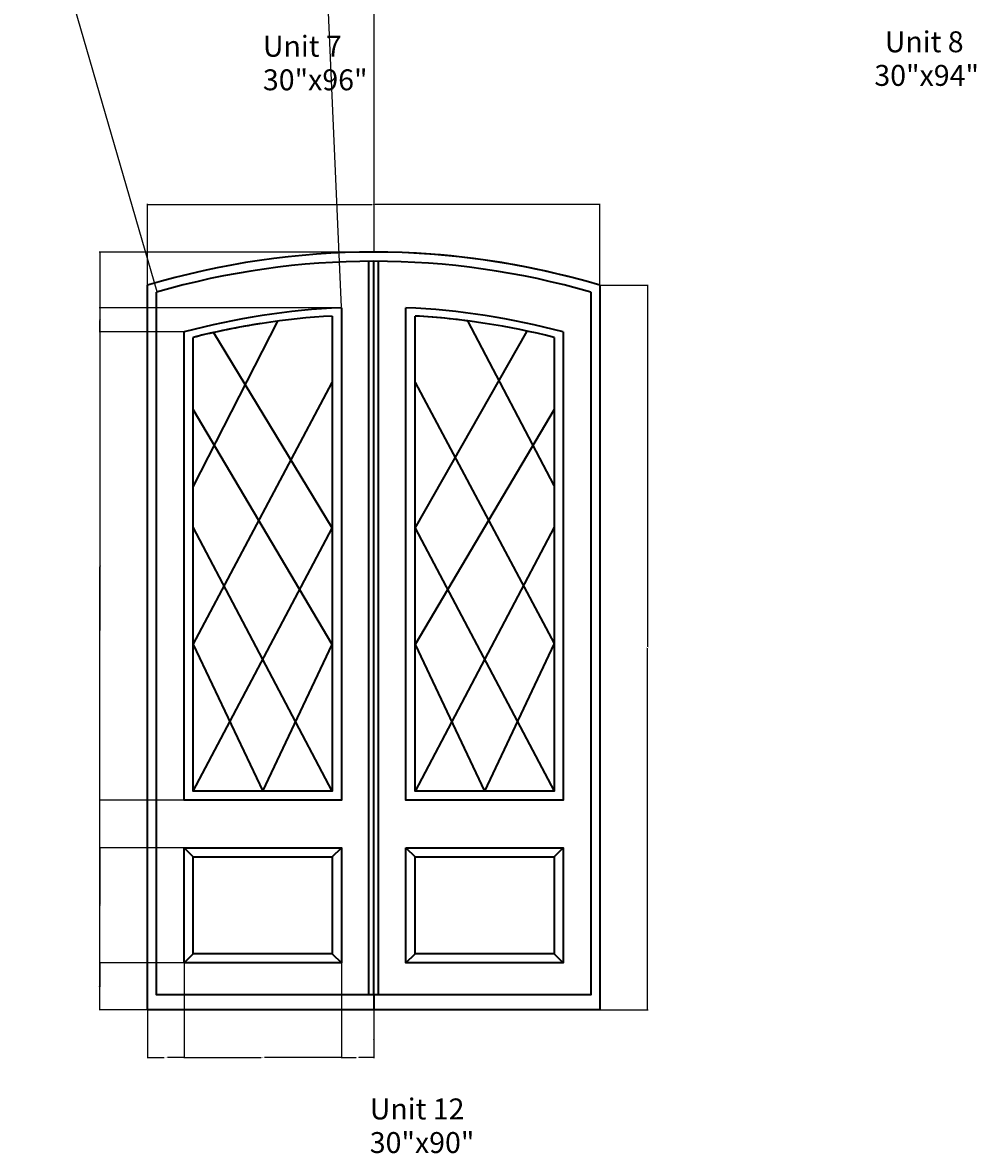
# Model space of a CAD drawing. Units: inches. Extents: x 1318 to 1980, y 617 to 1423.
# Tile 2 of 7: x 1656 to 1930, y 617 to 942. Entities that reach past the tile are written whole.
import ezdxf

# ---------------------------------------------------------------- set-up
doc = ezdxf.new("R2010")
doc.units = ezdxf.units.IN
doc.header["$MEASUREMENT"] = 0
for name, color, linetype, lineweight in [('A-ANNO-DIMS', 2, 'Continuous', 18), ('A-ANNO-TEXT', 7, 'Continuous', 25), ('A-DOOR', 4, 'Continuous', 35)]:
    doc.layers.add(name, color=color, linetype=linetype, lineweight=lineweight)
doc.styles.get("Standard").update_dxf_attribs({"font": 'arial.ttf'})
doc.dimstyles.get("Standard").update_dxf_attribs({"dimtxt": 0.18, "dimasz": 0.18, "dimexe": 0.18, "dimexo": 0.0625, "dimgap": 0.09, "dimtad": 0, "dimtih": 1, "dimtoh": 1, "dimdec": 0, "dimzin": 0, "dimdsep": 46, "dimlunit": 3, "dimtxsty": 'Standard', "dimcen": 0.09, "dimadec": 0, "dimazin": 0, "dimtfac": 1, "dimtdec": 0, "dimtofl": 0, "dimtmove": 0, "dimatfit": 3, "dimfxl": 1, "dimtolj": 1, "dimtzin": 0, "dimarcsym": 0})

# ---------------------------------------------------------------- blocks, each defined once
blk = doc.blocks.new('*D94')
at = {"layer": 'A-ANNO-DIMS', "color": 0, "lineweight": -2, "transparency": 16777216}
for p, q in [((1691.91, 866.32), (1691.91, 889.61)), ((1692.09, 889.43), (1756.33, 889.43)), ((1821.49, 889.43), (1757.24, 889.43)), ((1821.67, 866.32), (1821.67, 889.61))]:
    blk.add_line(p, q, dxfattribs=at)
at = {"layer": 'A-ANNO-DIMS', "color": 0, "transparency": 16777216}
for points in [[(1692.09, 889.46), (1692.09, 889.4), (1691.91, 889.43)], [(1821.49, 889.46), (1821.49, 889.4), (1821.67, 889.43)]]:
    blk.add_solid(points, dxfattribs=at)
at = {"layer": 'Defpoints', "color": 0, "transparency": 16777216}
for p in [(1821.67, 889.43), (1691.91, 866.26), (1821.67, 866.26)]:
    blk.add_point(p, dxfattribs=at)
at = {"layer": 'A-ANNO-DIMS', "color": 0, "transparency": 16777216, "insert": (1756.79, 889.43), "char_height": 0.18, "attachment_point": 5}
blk.add_mtext('\\A1;129.76', dxfattribs=at)
blk = doc.blocks.new('*D95')
at = {"layer": 'A-ANNO-DIMS', "color": 0, "lineweight": -2, "transparency": 16777216}
for p, q in [((1756.72, 875.78), (1678.08, 875.78)), ((1678.26, 875.6), (1678.26, 767.29)), ((1678.26, 658.62), (1678.26, 766.92)), ((1691.85, 658.44), (1678.08, 658.44))]:
    blk.add_line(p, q, dxfattribs=at)
at = {"layer": 'A-ANNO-DIMS', "color": 0, "transparency": 16777216}
for points in [[(1678.23, 875.6), (1678.29, 875.6), (1678.26, 875.78)], [(1678.23, 658.62), (1678.29, 658.62), (1678.26, 658.44)]]:
    blk.add_solid(points, dxfattribs=at)
at = {"layer": 'Defpoints', "color": 0, "transparency": 16777216}
for p in [(1678.26, 875.78), (1756.79, 875.78), (1691.91, 658.44)]:
    blk.add_point(p, dxfattribs=at)
at = {"layer": 'A-ANNO-DIMS', "color": 0, "transparency": 16777216, "insert": (1678.26, 767.11), "char_height": 0.18, "attachment_point": 5}
blk.add_mtext('\\A1;217.34', dxfattribs=at)
blk = doc.blocks.new('*D96')
at = {"layer": 'A-ANNO-DIMS', "color": 0, "lineweight": -2, "transparency": 16777216}
for p, q in [((1747.46, 859.84), (1678.08, 859.84)), ((1678.26, 859.66), (1678.26, 856.54)), ((1678.26, 853.06), (1678.26, 856.18)), ((1702.33, 852.88), (1678.08, 852.88))]:
    blk.add_line(p, q, dxfattribs=at)
at = {"layer": 'A-ANNO-DIMS', "color": 0, "transparency": 16777216}
for points in [[(1678.23, 859.66), (1678.29, 859.66), (1678.26, 859.84)], [(1678.23, 853.06), (1678.29, 853.06), (1678.26, 852.88)]]:
    blk.add_solid(points, dxfattribs=at)
at = {"layer": 'Defpoints', "color": 0, "transparency": 16777216}
for p in [(1678.26, 859.84), (1747.52, 859.84), (1702.4, 852.88)]:
    blk.add_point(p, dxfattribs=at)
at = {"layer": 'A-ANNO-DIMS', "color": 0, "transparency": 16777216, "insert": (1678.26, 856.36), "char_height": 0.18, "attachment_point": 5}
blk.add_mtext('\\A1;6.956', dxfattribs=at)
blk = doc.blocks.new('*D97')
at = {"layer": 'A-ANNO-DIMS', "color": 0, "lineweight": -2, "transparency": 16777216}
for p, q in [((1821.73, 866.26), (1835.5, 866.26)), ((1835.32, 866.08), (1835.32, 762.53)), ((1835.32, 658.62), (1835.32, 762.17)), ((1821.73, 658.44), (1835.5, 658.44))]:
    blk.add_line(p, q, dxfattribs=at)
at = {"layer": 'A-ANNO-DIMS', "color": 0, "transparency": 16777216}
for points in [[(1835.29, 866.08), (1835.35, 866.08), (1835.32, 866.26)], [(1835.29, 658.62), (1835.35, 658.62), (1835.32, 658.44)]]:
    blk.add_solid(points, dxfattribs=at)
at = {"layer": 'Defpoints', "color": 0, "transparency": 16777216}
for p in [(1821.67, 866.26), (1835.32, 866.26), (1821.67, 658.44)]:
    blk.add_point(p, dxfattribs=at)
at = {"layer": 'A-ANNO-DIMS', "color": 0, "transparency": 16777216, "insert": (1835.32, 762.35), "char_height": 0.18, "attachment_point": 5}
blk.add_mtext('\\A1;207.82', dxfattribs=at)
blk = doc.blocks.new('*D98')
at = {"layer": 'A-ANNO-DIMS', "color": 0, "lineweight": -2, "transparency": 16777216}
for p, q in [((1702.4, 671.85), (1702.4, 644.61)), ((1691.91, 658.37), (1691.91, 644.61)), ((1692.09, 644.79), (1696.7, 644.79)), ((1702.22, 644.79), (1697.61, 644.79))]:
    blk.add_line(p, q, dxfattribs=at)
at = {"layer": 'A-ANNO-DIMS', "color": 0, "transparency": 16777216}
for points in [[(1692.09, 644.82), (1692.09, 644.76), (1691.91, 644.79)], [(1702.22, 644.82), (1702.22, 644.76), (1702.4, 644.79)]]:
    blk.add_solid(points, dxfattribs=at)
at = {"layer": 'Defpoints', "color": 0, "transparency": 16777216}
for p in [(1702.4, 671.91), (1691.91, 658.44), (1702.4, 644.79)]:
    blk.add_point(p, dxfattribs=at)
at = {"layer": 'A-ANNO-DIMS', "color": 0, "transparency": 16777216, "insert": (1697.15, 644.79), "char_height": 0.18, "attachment_point": 5}
blk.add_mtext('\\A1;10.488', dxfattribs=at)
blk = doc.blocks.new('*D99')
at = {"layer": 'A-ANNO-DIMS', "color": 0, "lineweight": -2, "transparency": 16777216}
for p, q in [((1702.4, 671.85), (1702.4, 644.61)), ((1747.52, 671.85), (1747.52, 644.61)), ((1702.58, 644.79), (1724.49, 644.79)), ((1747.34, 644.79), (1725.43, 644.79))]:
    blk.add_line(p, q, dxfattribs=at)
at = {"layer": 'A-ANNO-DIMS', "color": 0, "transparency": 16777216}
for points in [[(1702.58, 644.82), (1702.58, 644.76), (1702.4, 644.79)], [(1747.34, 644.82), (1747.34, 644.76), (1747.52, 644.79)]]:
    blk.add_solid(points, dxfattribs=at)
at = {"layer": 'Defpoints', "color": 0, "transparency": 16777216}
for p in [(1702.4, 671.91), (1747.52, 671.91), (1747.52, 644.79)]:
    blk.add_point(p, dxfattribs=at)
at = {"layer": 'A-ANNO-DIMS', "color": 0, "transparency": 16777216, "insert": (1724.96, 644.79), "char_height": 0.18, "attachment_point": 5}
blk.add_mtext('\\A1;45.125', dxfattribs=at)
blk = doc.blocks.new('*D100')
at = {"layer": 'A-ANNO-DIMS', "color": 0, "lineweight": -2, "transparency": 16777216}
for p, q in [((1747.52, 671.85), (1747.52, 644.61)), ((1756.79, 658.37), (1756.79, 644.61)), ((1747.7, 644.79), (1751.76, 644.79)), ((1756.61, 644.79), (1752.55, 644.79))]:
    blk.add_line(p, q, dxfattribs=at)
at = {"layer": 'A-ANNO-DIMS', "color": 0, "transparency": 16777216}
for points in [[(1747.7, 644.82), (1747.7, 644.76), (1747.52, 644.79)], [(1756.61, 644.82), (1756.61, 644.76), (1756.79, 644.79)]]:
    blk.add_solid(points, dxfattribs=at)
at = {"layer": 'Defpoints', "color": 0, "transparency": 16777216}
for p in [(1747.52, 671.91), (1756.79, 658.44), (1756.79, 644.79)]:
    blk.add_point(p, dxfattribs=at)
at = {"layer": 'A-ANNO-DIMS', "color": 0, "transparency": 16777216, "insert": (1752.15, 644.79), "char_height": 0.18, "attachment_point": 5}
blk.add_mtext('\\A1;9.266', dxfattribs=at)
blk = doc.blocks.new('*D101')
at = {"layer": 'A-ANNO-DIMS', "color": 0, "lineweight": -2, "transparency": 16777216}
for p, q in [((1702.33, 671.91), (1678.08, 671.91)), ((1678.26, 671.73), (1678.26, 665.36)), ((1678.26, 658.62), (1678.26, 664.99)), ((1691.85, 658.44), (1678.08, 658.44))]:
    blk.add_line(p, q, dxfattribs=at)
at = {"layer": 'A-ANNO-DIMS', "color": 0, "transparency": 16777216}
for points in [[(1678.23, 671.73), (1678.29, 671.73), (1678.26, 671.91)], [(1678.23, 658.62), (1678.29, 658.62), (1678.26, 658.44)]]:
    blk.add_solid(points, dxfattribs=at)
at = {"layer": 'Defpoints', "color": 0, "transparency": 16777216}
for p in [(1678.26, 671.91), (1702.4, 671.91), (1691.91, 658.44)]:
    blk.add_point(p, dxfattribs=at)
at = {"layer": 'A-ANNO-DIMS', "color": 0, "transparency": 16777216, "insert": (1678.26, 665.17), "char_height": 0.18, "attachment_point": 5}
blk.add_mtext('\\A1;13.477', dxfattribs=at)
blk = doc.blocks.new('*D102')
at = {"layer": 'A-ANNO-DIMS', "color": 0, "lineweight": -2, "transparency": 16777216}
for p, q in [((1702.33, 704.96), (1678.08, 704.96)), ((1678.26, 704.78), (1678.26, 688.62)), ((1678.26, 672.09), (1678.26, 688.25)), ((1702.33, 671.91), (1678.08, 671.91))]:
    blk.add_line(p, q, dxfattribs=at)
at = {"layer": 'A-ANNO-DIMS', "color": 0, "transparency": 16777216}
for points in [[(1678.23, 704.78), (1678.29, 704.78), (1678.26, 704.96)], [(1678.23, 672.09), (1678.29, 672.09), (1678.26, 671.91)]]:
    blk.add_solid(points, dxfattribs=at)
at = {"layer": 'Defpoints', "color": 0, "transparency": 16777216}
for p in [(1678.26, 704.96), (1702.4, 704.96), (1702.4, 671.91)]:
    blk.add_point(p, dxfattribs=at)
at = {"layer": 'A-ANNO-DIMS', "color": 0, "transparency": 16777216, "insert": (1678.26, 688.44), "char_height": 0.18, "attachment_point": 5}
blk.add_mtext('\\A1;33.046', dxfattribs=at)
blk = doc.blocks.new('*D103')
at = {"layer": 'A-ANNO-DIMS', "color": 0, "lineweight": -2, "transparency": 16777216}
for p, q in [((1702.33, 852.88), (1678.08, 852.88)), ((1678.26, 852.7), (1678.26, 785.91)), ((1678.26, 718.75), (1678.26, 785.55)), ((1702.33, 718.57), (1678.08, 718.57))]:
    blk.add_line(p, q, dxfattribs=at)
at = {"layer": 'A-ANNO-DIMS', "color": 0, "transparency": 16777216}
for points in [[(1678.23, 852.7), (1678.29, 852.7), (1678.26, 852.88)], [(1678.23, 718.75), (1678.29, 718.75), (1678.26, 718.57)]]:
    blk.add_solid(points, dxfattribs=at)
at = {"layer": 'Defpoints', "color": 0, "transparency": 16777216}
for p in [(1678.26, 852.88), (1702.4, 852.88), (1702.4, 718.57)]:
    blk.add_point(p, dxfattribs=at)
at = {"layer": 'A-ANNO-DIMS', "color": 0, "transparency": 16777216, "insert": (1678.26, 785.73), "char_height": 0.18, "attachment_point": 5}
blk.add_mtext('\\A1;134.3', dxfattribs=at)
blk = doc.blocks.new('*D118')
at = {"layer": 'A-ANNO-DIMS', "color": 0, "lineweight": -2, "transparency": 16777216}
for p, q in [((1756.97, 1011.3), (1756.79, 1011.3)), ((1756.79, 1011.3), (1756.79, 875.96)), ((1756.7, 649.9), (1756.88, 649.9)), ((1756.79, 649.81), (1756.79, 649.99))]:
    blk.add_line(p, q, dxfattribs=at)
at = {"layer": 'A-ANNO-DIMS', "color": 0, "transparency": 16777216}
blk.add_solid([(1756.76, 875.96), (1756.82, 875.96), (1756.79, 875.78)], dxfattribs=at)
at = {"layer": 'Defpoints', "color": 0, "transparency": 16777216}
for p in [(1756.79, 875.78), (1756.79, 649.9)]:
    blk.add_point(p, dxfattribs=at)
at = {"layer": 'A-ANNO-DIMS', "color": 0, "transparency": 16777216, "insert": (1757.45, 1011.3), "char_height": 0.18, "attachment_point": 5}
blk.add_mtext('\\A1;R225.9', dxfattribs=at)
blk = doc.blocks.new('*D119')
at = {"layer": 'A-ANNO-DIMS', "color": 0, "lineweight": -2, "transparency": 16777216}
for p, q in [((1657.1, 992.97), (1657.28, 992.97)), ((1657.28, 992.97), (1694.55, 864.49)), ((1756.7, 649.9), (1756.88, 649.9)), ((1756.79, 649.81), (1756.79, 649.99))]:
    blk.add_line(p, q, dxfattribs=at)
at = {"layer": 'A-ANNO-DIMS', "color": 0, "transparency": 16777216}
blk.add_solid([(1694.57, 864.5), (1694.52, 864.48), (1694.6, 864.32)], dxfattribs=at)
at = {"layer": 'Defpoints', "color": 0, "transparency": 16777216}
for p in [(1694.6, 864.32), (1756.79, 649.9)]:
    blk.add_point(p, dxfattribs=at)
at = {"layer": 'A-ANNO-DIMS', "color": 0, "transparency": 16777216, "insert": (1656.55, 992.97), "char_height": 0.18, "attachment_point": 5}
blk.add_mtext('\\A1;R223.26', dxfattribs=at)
blk = doc.blocks.new('*D120')
at = {"layer": 'A-ANNO-DIMS', "color": 0, "lineweight": -2, "transparency": 16777216}
for p, q in [((1741.75, 985.8), (1741.93, 985.8)), ((1741.93, 985.8), (1747.49, 860.02)), ((1756.7, 649.9), (1756.88, 649.9)), ((1756.79, 649.81), (1756.79, 649.99))]:
    blk.add_line(p, q, dxfattribs=at)
at = {"layer": 'A-ANNO-DIMS', "color": 0, "transparency": 16777216}
blk.add_solid([(1747.52, 860.02), (1747.46, 860.02), (1747.5, 859.84)], dxfattribs=at)
at = {"layer": 'Defpoints', "color": 0, "transparency": 16777216}
for p in [(1747.5, 859.84), (1756.79, 649.9)]:
    blk.add_point(p, dxfattribs=at)
at = {"layer": 'A-ANNO-DIMS', "color": 0, "transparency": 16777216, "insert": (1741, 985.8), "char_height": 0.18, "attachment_point": 5}
blk.add_mtext('\\A1;4X R210.15', dxfattribs=at)

msp = doc.modelspace()

# ---------------------------------------------------------------- linework, layer by layer
at = {"layer": 'A-DOOR'}
for p, q in [((1755.3874, 662.7536), (1755.3874, 873.1492)), ((1756.7874, 662.7536), (1756.7874, 873.1536)), ((1758.1875, 662.7536), (1758.1875, 873.1492)), ((1705.0189, 808.4828), (1729.2992, 855.9901)), ((1768.6751, 796.5833), (1800.8603, 853.1222)), ((1808.5559, 808.8309), (1783.7627, 856.0572)), ((1710.8281, 852.7085), (1744.8997, 796.5833)), ((1705.0189, 763.193), (1744.8997, 838.3489)), ((1768.6751, 838.3489), (1808.5559, 763.5027)), ((1744.8997, 763.193), (1705.0189, 830.6119)), ((1808.5559, 830.6119), (1768.6751, 763.193)), ((1744.8997, 721.1955), (1705.0189, 796.9217)), ((1705.0189, 721.1955), (1744.8997, 796.5833)), ((1808.5559, 796.9217), (1768.6751, 721.1955)), ((1768.6751, 796.5833), (1808.5559, 721.1955)), ((1705.0189, 763.193), (1724.9593, 721.1955)), ((1724.9593, 721.1955), (1744.8997, 763.193)), ((1768.6751, 763.193), (1788.6155, 721.1955)), ((1808.5559, 763.5027), (1788.6155, 721.1955)), ((1702.397, 704.9593), (1705.0189, 702.3374)), ((1744.8997, 702.3374), (1747.5217, 704.9593)), ((1766.0532, 704.9593), (1768.6751, 702.3374)), ((1808.5559, 702.3374), (1811.1778, 704.9593)), ((1702.397, 671.9133), (1705.0189, 674.5352)), ((1744.8997, 674.5352), (1747.5217, 671.9133)), ((1766.0532, 671.9133), (1768.6751, 674.5352)), ((1808.5559, 674.5352), (1811.1778, 671.9133)), ((1756.7874, 662.7536), (1756.7874, 658.4362))]:
    msp.add_line(p, q, dxfattribs=at)
for points in [[(1821.6654, 866.2577), (1821.6654, 658.4362), (1691.9094, 658.4362), (1691.9094, 866.2577)], [(1819.0435, 864.2978), (1819.0435, 662.7536), (1694.5313, 662.7536), (1694.5313, 864.2978)], [(1747.5217, 859.8397), (1747.5217, 718.5736), (1702.397, 718.5736), (1702.397, 852.8834)], [(1811.1778, 852.8834), (1811.1778, 718.5736), (1766.0532, 718.5736), (1766.0532, 859.8397)], [(1744.8997, 857.4592), (1744.8997, 721.1955), (1705.0189, 721.1955), (1705.0189, 851.3195)], [(1808.5559, 851.3195), (1808.5559, 721.1955), (1768.6751, 721.1955), (1768.6751, 857.4592)]]:
    msp.add_lwpolyline(points, dxfattribs=at)
for points in [[(1702.397, 704.9593), (1747.5217, 704.9593), (1747.5217, 671.9133), (1702.397, 671.9133)], [(1766.0532, 704.9593), (1811.1778, 704.9593), (1811.1778, 671.9133), (1766.0532, 671.9133)], [(1705.0189, 702.3374), (1744.8997, 702.3374), (1744.8997, 674.5352), (1705.0189, 674.5352)], [(1768.6751, 702.3374), (1808.5559, 702.3374), (1808.5559, 674.5352), (1768.6751, 674.5352)]]:
    msp.add_lwpolyline(points, close=True, dxfattribs=at)
for centre, radius, start, end in [((1756.7874, 649.8957), 225.8798, 73.308188, 106.691812), ((1756.7874, 649.8957), 223.2579, 73.808245, 106.191755), ((1756.7874, 649.8957), 225.8798, 75, 87.472922), ((1756.7874, 649.8957), 210.1484, 92.527078, 105), ((1756.7874, 649.8957), 210.1484, 75, 87.472922), ((1756.7874, 647.6473), 210.1484, 93.242837, 104.261191), ((1756.7874, 647.6473), 210.1484, 75.738809, 86.757163), ((1756.7874, 647.6473), 210.1484, 81.431136, 86.757163), ((1756.7874, 647.6473), 210.1484, 98.853734, 104.261191)]:
    msp.add_arc(centre, radius, start, end, dxfattribs=at)

# ---------------------------------------------------------------- texts
at = {"layer": 'A-ANNO-TEXT'}
for s, p in [('Unit 7', (1725.0196, 931.8396)), ('Unit 8', (1903.3865, 933.11)), ('30"x96"', (1725.0196, 922.2011)), ('30"x94"', (1900.3947, 923.4715)), ('Unit 12', (1755.6667, 627.0252)), ('30"x90"', (1755.6667, 617.3867))]:
    msp.add_text(s, height=6, dxfattribs=at).set_placement(p)

# ---------------------------------------------------------------- dimensions: what is measured, and where the dimension line sits
at = {"layer": 'A-ANNO-DIMS'}
for mpoint, override, picture, middle in [((1756.79, 875.7755), {"dimdec": 1, "dimlfac": 1, "dimrnd": 0, "dimzin": 0, "dimdsep": 46, "dimlunit": 2}, '*D118', (1757.4516, 1011.3033)), ((1694.5953, 864.3163), {"dimdec": 2, "dimlfac": 1, "dimrnd": 0, "dimzin": 0, "dimdsep": 46, "dimlunit": 2}, '*D119', (1656.5503, 992.9687))]:
    dim = msp.add_radius_dim(center=(1756.7874, 649.8957), mpoint=mpoint, dimstyle='Standard', override=override, dxfattribs=at)
    dim.commit()
    dim.dimension.update_dxf_attribs({"geometry": picture, "text_midpoint": middle, "dimtype": 164})
dim = msp.add_radius_dim(center=(1756.7874, 649.8957), mpoint=(1747.5027, 859.8388), text='4X <>', dimstyle='Standard', override={"dimdec": 2, "dimlfac": 1, "dimrnd": 0, "dimzin": 0, "dimdsep": 46, "dimlunit": 2}, dxfattribs=at)
dim.commit()
dim.dimension.update_dxf_attribs({"geometry": '*D120', "text_midpoint": (1741.0044, 985.8047), "dimtype": 164})
for base, p1, p2, override, picture, middle in [((1821.6654, 889.4255), (1691.9094, 866.2577), (1821.6654, 866.2577), {"dimdec": 2, "dimlfac": 1, "dimrnd": 0, "dimzin": 0, "dimdsep": 46, "dimlunit": 2}, '*D94', (1756.7874, 889.4255)), ((1702.397, 644.7862), (1691.9094, 658.4362), (1702.397, 671.9133), {"dimdec": 3, "dimlfac": 1, "dimrnd": 0, "dimzin": 0, "dimdsep": 46, "dimlunit": 2}, '*D98', (1697.1532, 644.7862)), ((1747.5217, 644.7862), (1702.397, 671.9133), (1747.5217, 671.9133), {"dimdec": 3, "dimlfac": 1, "dimrnd": 0, "dimzin": 0, "dimdsep": 46, "dimlunit": 2}, '*D99', (1724.9593, 644.7862)), ((1756.7874, 644.7862), (1747.5217, 671.9133), (1756.7874, 658.4362), {"dimdec": 3, "dimlfac": 1, "dimrnd": 0, "dimzin": 0, "dimdsep": 46, "dimlunit": 2}, '*D100', (1752.1545, 644.7862))]:
    dim = msp.add_linear_dim(base=base, p1=p1, p2=p2, dimstyle='Standard', override=override, dxfattribs=at)
    dim.commit()
    dim.dimension.update_dxf_attribs({"geometry": picture, "text_midpoint": middle})
for base, p1, p2, override, picture, middle in [((1678.2594, 875.7755), (1691.9094, 658.4362), (1756.7874, 875.7755), {"dimdec": 2, "dimlfac": 1, "dimrnd": 0, "dimzin": 0, "dimdsep": 46, "dimlunit": 2}, '*D95', (1678.2594, 767.1059)), ((1835.3154, 866.2577), (1821.6654, 658.4362), (1821.6654, 866.2577), {"dimdec": 2, "dimlfac": 1, "dimrnd": 0, "dimzin": 0, "dimdsep": 46, "dimlunit": 2}, '*D97', (1835.3154, 762.347)), ((1678.2594, 859.8397), (1702.397, 852.8834), (1747.5217, 859.8397), {"dimdec": 3, "dimlfac": 1, "dimrnd": 0, "dimzin": 0, "dimdsep": 46, "dimlunit": 2}, '*D96', (1678.2594, 856.3615)), ((1678.2594, 852.8834), (1702.397, 718.5736), (1702.397, 852.8834), {"dimdec": 1, "dimlfac": 1, "dimrnd": 0, "dimzin": 0, "dimdsep": 46, "dimlunit": 2}, '*D103', (1678.2594, 785.7285)), ((1678.2594, 704.9593), (1702.397, 671.9133), (1702.397, 704.9593), {"dimdec": 3, "dimlfac": 1, "dimrnd": 0, "dimzin": 0, "dimdsep": 46, "dimlunit": 2}, '*D102', (1678.2594, 688.4363)), ((1678.2594, 671.9133), (1691.9094, 658.4362), (1702.397, 671.9133), {"dimdec": 3, "dimlfac": 1, "dimrnd": 0, "dimzin": 0, "dimdsep": 46, "dimlunit": 2}, '*D101', (1678.2594, 665.1748))]:
    dim = msp.add_linear_dim(base=base, p1=p1, p2=p2, angle=90, dimstyle='Standard', override=override, dxfattribs=at)
    dim.commit()
    dim.dimension.update_dxf_attribs({"geometry": picture, "text_midpoint": middle})

doc.saveas('drawing.dxf')
